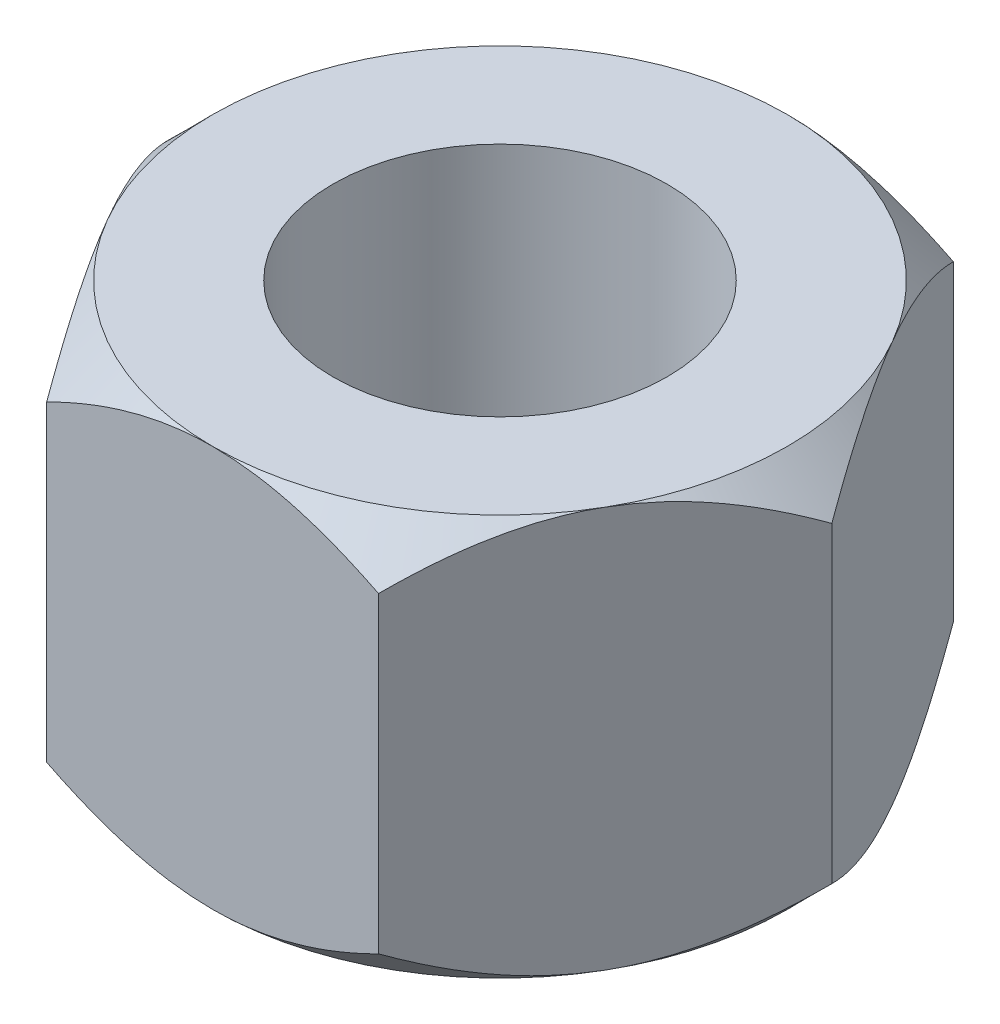
from build123d import *

# Parameters (mm, degrees)
HEX_BODY_3MM_DEPTH              = 3
FACE_CHAMFER_A_SKETCH_OUTSIDE_W = 14.41
FACE_CHAMFER_A_SKETCH_OUTSIDE_H = 13.744
FACE_CHAMFER_A_SKETCH_OUTSIDE_R = 2.15
FACE_CHAMFER_A_45DEG_DEPTH      = 3
FACE_CHAMFER_A_45DEG_DRAFT      = -45
FACE_CHAMFER_B_SKETCH_OUTSIDE_W = 14.41
FACE_CHAMFER_B_SKETCH_OUTSIDE_H = 13.744
FACE_CHAMFER_B_SKETCH_OUTSIDE_R = 2.15
FACE_CHAMFER_B_45DEG_DEPTH      = 3
FACE_CHAMFER_B_45DEG_DRAFT      = -45
BORE_2_5_SKETCH_R               = 1.25
THROUGH_BORE_2_5_DEPTH          = 23


with BuildPart() as part:
    # Hex Profile 4.3AF Sketch → Hex Body 3mm (new body)
    with BuildSketch(Plane(origin=(0, 0, 0), x_dir=(1, 0, 0), z_dir=(0, 1, 0))):
        Polygon((1.241303079, -2.15), (2.482606158, 0), (1.241303079, 2.15), (-1.241303079, 2.15), (-2.482606158, 0), (-1.241303079, -2.15), align=None)
    extrude(amount=HEX_BODY_3MM_DEPTH)


with BuildPart() as face_chamfer_a_45deg_tool:
    # Face Chamfer A Sketch outside → Face Chamfer A 45deg (with draft: the straight prism first)
    with BuildSketch(Plane(origin=(0, 3, 0), x_dir=(1, 0, 0), z_dir=(0, 1, 0))):
        Rectangle(FACE_CHAMFER_A_SKETCH_OUTSIDE_W, FACE_CHAMFER_A_SKETCH_OUTSIDE_H)
        Circle(FACE_CHAMFER_A_SKETCH_OUTSIDE_R, mode=Mode.SUBTRACT)
    extrude(amount=-FACE_CHAMFER_A_45DEG_DEPTH)
    # Face Chamfer A 45deg: the draft: its side faces are tilted about the plane it starts from
    face_chamfer_a_45deg_sides = [face_chamfer_a_45deg_tool.faces().sort_by_distance(p)[0] for p in [
        (0, 1.5, 6.872),
        (7.205, 1.5, 0),
        (0, 1.5, -6.872),
        (-7.205, 1.5, 0),
        (-2.15, 1.5, 0),
    ]]
    draft(face_chamfer_a_45deg_sides, Plane(origin=(0, 3, 0), x_dir=(1, 0, 0), z_dir=(0, 1, 0)), FACE_CHAMFER_A_45DEG_DRAFT)


with BuildPart() as part_1:
    add(part.part)

    # Face Chamfer A 45deg: cut by face_chamfer_a_45deg_tool
    add(face_chamfer_a_45deg_tool.part, mode=Mode.SUBTRACT)


with BuildPart() as face_chamfer_b_45deg_tool:
    # Face Chamfer B Sketch outside → Face Chamfer B 45deg (with draft: the straight prism first)
    with BuildSketch(Plane.XZ):
        Rectangle(FACE_CHAMFER_B_SKETCH_OUTSIDE_W, FACE_CHAMFER_B_SKETCH_OUTSIDE_H)
        Circle(FACE_CHAMFER_B_SKETCH_OUTSIDE_R, mode=Mode.SUBTRACT)
    extrude(amount=-FACE_CHAMFER_B_45DEG_DEPTH)
    # Face Chamfer B 45deg: the draft: its side faces are tilted about the plane it starts from
    face_chamfer_b_45deg_sides = [face_chamfer_b_45deg_tool.faces().sort_by_distance(p)[0] for p in [
        (0, 1.5, -6.872),
        (7.205, 1.5, 0),
        (0, 1.5, 6.872),
        (-7.205, 1.5, 0),
        (-2.15, 1.5, 0),
    ]]
    draft(face_chamfer_b_45deg_sides, Plane.XZ, FACE_CHAMFER_B_45DEG_DRAFT)


with BuildPart() as part_2:
    add(part_1.part)

    # Face Chamfer B 45deg: cut by face_chamfer_b_45deg_tool
    add(face_chamfer_b_45deg_tool.part, mode=Mode.SUBTRACT)

    # Bore Ø2.5 Sketch → Through Bore Ø2.5 (cut)
    with BuildSketch(Plane.XZ):
        with Locations(Location((0, 0, 0), (0, 0, 270))):
            Circle(BORE_2_5_SKETCH_R)
    extrude(amount=-THROUGH_BORE_2_5_DEPTH, mode=Mode.SUBTRACT)


solid = part_2.part
